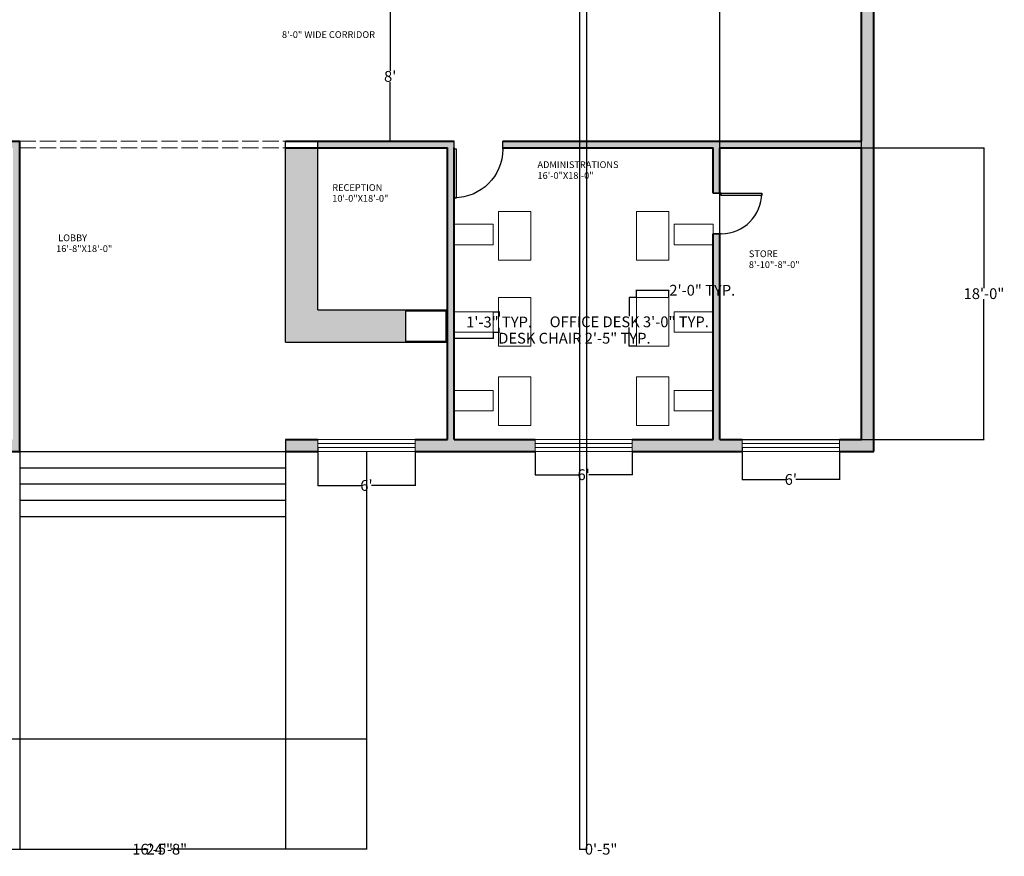
# Model space of a CAD drawing. Units: inches. Extents: x -405 to 940, y 226 to 2032.
# Tile 2 of 10: x 183 to 913, y 226 to 846. Entities that reach past the tile are written whole.
import ezdxf

# ---------------------------------------------------------------- set-up
doc = ezdxf.new("R2010")
doc.units = ezdxf.units.IN
doc.header["$MEASUREMENT"] = 0
doc.linetypes.add('ACAD_ISO02W100', pattern=[15, 12, -3])
for name, color, linetype, lineweight in [('A-ANNO-DIMS', 120, 'Continuous', 18), ('A-AREA-IDEN', 32, 'Continuous', 18), ('A-DOOR-OVHD', 6, 'ACAD_ISO02W100', 18), ('A-FLOR-CASE', 3, 'Continuous', 30), ('A-FLOR-EDGE', 3, 'Continuous', 25), ('A-FURN-SEAT', 5, 'Continuous', 18), ('A-GLAZ-HIDN', 1, 'ACAD_ISO02W100', 18), ('A-WALL-PATT', 8, 'Continuous', 13), ('door', 6, 'Continuous', 25), ('stair', 38, 'Continuous', 25), ('tables', 2, 'Continuous', 18), ('wall', 3, 'Continuous', 40), ('window', 1, 'Continuous', 18)]:
    doc.layers.add(name, color=color, linetype=linetype, lineweight=lineweight)
doc.styles.get("Standard").update_dxf_attribs({"font": 'arial.ttf'})
doc.dimstyles.get("Standard").update_dxf_attribs({"dimtxt": 8, "dimasz": 0.18, "dimexe": 0.18, "dimexo": 0.0625, "dimgap": 0.09, "dimtad": 0, "dimtih": 1, "dimtoh": 1, "dimdec": 0, "dimzin": 0, "dimdsep": 46, "dimlunit": 3, "dimtxsty": 'Standard', "dimblk": 'OBLIQUE', "dimcen": 0.09, "dimadec": 0, "dimazin": 0, "dimtfac": 1, "dimtdec": 0, "dimtofl": 0, "dimtmove": 0, "dimatfit": 3, "dimfxl": 1, "dimtolj": 1, "dimtzin": 0, "dimarcsym": 0})

# ---------------------------------------------------------------- blocks, each defined once
blk = doc.blocks.new('*U3')
for p, q in [((0, 0), (0, -6)), ((30, 0), (30, -6))]:
    blk.add_line(p, q)
blk.add_lwpolyline([(0, 0), (0, 30), (1.75, 30), (1.75, 0)], close=True)
blk.add_arc((0, 0), 30, 0, 90)
blk = doc.blocks.new('*U4')
for p, q in [((0, 0), (0, -6)), ((36, 0), (36, -6))]:
    blk.add_line(p, q)
blk.add_lwpolyline([(0, 0), (0, 36), (1.75, 36), (1.75, 0)], close=True)
blk.add_arc((0, 0), 36, 0, 90)
blk = doc.blocks.new('_Oblique')
at = {"color": 0, "linetype": 'ByBlock', "lineweight": -2}
blk.add_line((-0.5, -0.5), (0.5, 0.5), dxfattribs=at)
blk = doc.blocks.new('*D39')
at = {"layer": 'A-ANNO-DIMS', "color": 0, "lineweight": -2, "transparency": 16777216}
for p, q in [((460.94, 851.81), (457.18, 851.81)), ((457.36, 851.81), (457.36, 807.98)), ((457.36, 755.81), (457.36, 799.64)), ((460.94, 755.81), (457.18, 755.81))]:
    blk.add_line(p, q, dxfattribs=at)
at = {"layer": 'Defpoints', "color": 0, "transparency": 16777216}
for p in [(457.36, 851.81), (461, 851.81), (461, 755.81)]:
    blk.add_point(p, dxfattribs=at)
at = {"layer": 'A-ANNO-DIMS', "color": 0, "lineweight": -2, "transparency": 16777216, "xscale": 0.18, "yscale": 0.18, "zscale": 0.18}
for p, rotation in [((457.36, 851.81), 90), ((457.36, 755.81), 270)]:
    blk.add_blockref('_Oblique', p, dxfattribs=dict(at, rotation=rotation))
at = {"layer": 'A-ANNO-DIMS', "color": 0, "transparency": 16777216, "insert": (457.36, 803.81), "char_height": 8, "attachment_point": 5}
blk.add_mtext("\\A1;8'", dxfattribs=at)
blk = doc.blocks.new('*D72')
at = {"layer": 'A-ANNO-DIMS', "color": 0, "lineweight": -2, "transparency": 16777216}
for p, q in [((718.27, 528.75), (718.27, 504.97)), ((790.27, 525.75), (790.27, 504.97)), ((718.27, 505.15), (750.48, 505.15)), ((790.27, 505.15), (758.06, 505.15))]:
    blk.add_line(p, q, dxfattribs=at)
at = {"layer": 'Defpoints', "color": 0, "transparency": 16777216}
for p in [(718.27, 528.81), (790.27, 525.81), (718.27, 505.15)]:
    blk.add_point(p, dxfattribs=at)
at = {"layer": 'A-ANNO-DIMS', "color": 0, "lineweight": -2, "transparency": 16777216, "xscale": 0.18, "yscale": 0.18, "zscale": 0.18, "rotation": 180}
blk.add_blockref('_Oblique', (718.27, 505.15), dxfattribs=at)
at = {"layer": 'A-ANNO-DIMS', "color": 0, "lineweight": -2, "transparency": 16777216, "xscale": 0.18, "yscale": 0.18, "zscale": 0.18}
blk.add_blockref('_Oblique', (790.27, 505.15), dxfattribs=at)
at = {"layer": 'A-ANNO-DIMS', "color": 0, "transparency": 16777216, "insert": (754.27, 505.15), "char_height": 8, "attachment_point": 5}
blk.add_mtext("\\A1;6'", dxfattribs=at)
blk = doc.blocks.new('*D73')
at = {"layer": 'A-ANNO-DIMS', "color": 0, "lineweight": -2, "transparency": 16777216}
for p, q in [((564.77, 525.75), (564.77, 508.48)), ((636.77, 525.75), (636.77, 508.48)), ((564.77, 508.66), (596.98, 508.66)), ((636.77, 508.66), (604.56, 508.66))]:
    blk.add_line(p, q, dxfattribs=at)
at = {"layer": 'Defpoints', "color": 0, "transparency": 16777216}
for p in [(564.77, 525.81), (636.77, 525.81), (636.77, 508.66)]:
    blk.add_point(p, dxfattribs=at)
at = {"layer": 'A-ANNO-DIMS', "color": 0, "lineweight": -2, "transparency": 16777216, "xscale": 0.18, "yscale": 0.18, "zscale": 0.18, "rotation": 180}
blk.add_blockref('_Oblique', (564.77, 508.66), dxfattribs=at)
at = {"layer": 'A-ANNO-DIMS', "color": 0, "lineweight": -2, "transparency": 16777216, "xscale": 0.18, "yscale": 0.18, "zscale": 0.18}
blk.add_blockref('_Oblique', (636.77, 508.66), dxfattribs=at)
at = {"layer": 'A-ANNO-DIMS', "color": 0, "transparency": 16777216, "insert": (600.77, 508.66), "char_height": 8, "attachment_point": 5}
blk.add_mtext("\\A1;6'", dxfattribs=at)
blk = doc.blocks.new('*D74')
at = {"layer": 'A-ANNO-DIMS', "color": 0, "lineweight": -2, "transparency": 16777216}
for p, q in [((403.77, 528.75), (403.77, 500.53)), ((475.77, 525.75), (475.77, 500.53)), ((403.77, 500.71), (435.98, 500.71)), ((475.77, 500.71), (443.56, 500.71))]:
    blk.add_line(p, q, dxfattribs=at)
at = {"layer": 'Defpoints', "color": 0, "transparency": 16777216}
for p in [(403.77, 528.81), (475.77, 525.81), (475.77, 500.71)]:
    blk.add_point(p, dxfattribs=at)
at = {"layer": 'A-ANNO-DIMS', "color": 0, "lineweight": -2, "transparency": 16777216, "xscale": 0.18, "yscale": 0.18, "zscale": 0.18, "rotation": 180}
blk.add_blockref('_Oblique', (403.77, 500.71), dxfattribs=at)
at = {"layer": 'A-ANNO-DIMS', "color": 0, "lineweight": -2, "transparency": 16777216, "xscale": 0.18, "yscale": 0.18, "zscale": 0.18}
blk.add_blockref('_Oblique', (475.77, 500.71), dxfattribs=at)
at = {"layer": 'A-ANNO-DIMS', "color": 0, "transparency": 16777216, "insert": (439.77, 500.71), "char_height": 8, "attachment_point": 5}
blk.add_mtext("\\A1;6'", dxfattribs=at)
blk = doc.blocks.new('DESK-24X36IN')
for p, q in [((0, 36), (24, 36)), ((0, 0), (0, 36)), ((24, 36), (24, 0)), ((24, 0), (0, 0))]:
    blk.add_line(p, q)
blk = doc.blocks.new('CHAIR-DESK')
blk.add_lwpolyline([(0, 15.21), (28.97, 15.21), (28.97, 0), (0, 0)], close=True)
blk = doc.blocks.new('WIN-PANE-72IN')
for p, q in [((0, 3), (72, 3)), ((0, 0), (72, 0))]:
    blk.add_line(p, q)
blk = doc.blocks.new('*D87')
at = {"layer": 'A-ANNO-DIMS', "color": 0, "lineweight": -2, "transparency": 16777216}
for p, q in [((504.77, 614.1), (504.77, 609.63)), ((533.73, 614.1), (533.73, 609.63)), ((504.77, 609.81), (533.73, 609.81)), ((533.73, 609.81), (533.91, 609.81))]:
    blk.add_line(p, q, dxfattribs=at)
at = {"layer": 'Defpoints', "color": 0, "transparency": 16777216}
for p in [(504.77, 614.16), (533.73, 614.16), (533.73, 609.81)]:
    blk.add_point(p, dxfattribs=at)
at = {"layer": 'A-ANNO-DIMS', "color": 0, "lineweight": -2, "transparency": 16777216, "xscale": 0.18, "yscale": 0.18, "zscale": 0.18, "rotation": 180}
blk.add_blockref('_Oblique', (504.77, 609.81), dxfattribs=at)
at = {"layer": 'A-ANNO-DIMS', "color": 0, "lineweight": -2, "transparency": 16777216, "xscale": 0.18, "yscale": 0.18, "zscale": 0.18}
blk.add_blockref('_Oblique', (533.73, 609.81), dxfattribs=at)
at = {"layer": 'A-ANNO-DIMS', "color": 0, "transparency": 16777216, "insert": (593.9, 609.81), "char_height": 8, "attachment_point": 5}
blk.add_mtext('\\A1;DESK CHAIR 2\'-5" TYP.', dxfattribs=at)
blk = doc.blocks.new('*D88')
at = {"layer": 'A-ANNO-DIMS', "color": 0, "lineweight": -2, "transparency": 16777216}
for p, q in [((533.8, 629.37), (538.26, 629.37)), ((538.08, 629.37), (538.08, 625.94)), ((533.8, 614.16), (538.26, 614.16)), ((538.08, 614.16), (538.08, 617.59))]:
    blk.add_line(p, q, dxfattribs=at)
at = {"layer": 'Defpoints', "color": 0, "transparency": 16777216}
for p in [(533.73, 629.37), (538.08, 629.37), (533.73, 614.16)]:
    blk.add_point(p, dxfattribs=at)
at = {"layer": 'A-ANNO-DIMS', "color": 0, "lineweight": -2, "transparency": 16777216, "xscale": 0.18, "yscale": 0.18, "zscale": 0.18}
for p, rotation in [((538.08, 629.37), 90), ((538.08, 614.16), 270)]:
    blk.add_blockref('_Oblique', p, dxfattribs=dict(at, rotation=rotation))
at = {"layer": 'A-ANNO-DIMS', "color": 0, "transparency": 16777216, "insert": (538.08, 621.77), "char_height": 8, "attachment_point": 5}
blk.add_mtext('\\A1;1\'-3" TYP.', dxfattribs=at)
blk = doc.blocks.new('*D89')
at = {"layer": 'A-ANNO-DIMS', "color": 0, "lineweight": -2, "transparency": 16777216}
for p, q in [((639.86, 639.95), (634.35, 639.95)), ((634.53, 639.95), (634.53, 626.19)), ((634.53, 603.95), (634.53, 617.72)), ((639.86, 603.95), (634.35, 603.95))]:
    blk.add_line(p, q, dxfattribs=at)
at = {"layer": 'Defpoints', "color": 0, "transparency": 16777216}
for p in [(634.53, 639.95), (639.93, 639.95), (639.93, 603.95)]:
    blk.add_point(p, dxfattribs=at)
at = {"layer": 'A-ANNO-DIMS', "color": 0, "lineweight": -2, "transparency": 16777216, "xscale": 0.18, "yscale": 0.18, "zscale": 0.18}
for p, rotation in [((634.53, 639.95), 90), ((634.53, 603.95), 270)]:
    blk.add_blockref('_Oblique', p, dxfattribs=dict(at, rotation=rotation))
at = {"layer": 'A-ANNO-DIMS', "color": 0, "transparency": 16777216, "insert": (634.53, 621.95), "char_height": 8, "attachment_point": 5}
blk.add_mtext('\\A1;OFFICE DESK 3\'-0" TYP.', dxfattribs=at)
blk = doc.blocks.new('*D90')
at = {"layer": 'A-ANNO-DIMS', "color": 0, "lineweight": -2, "transparency": 16777216}
for p, q in [((639.93, 640.02), (639.93, 645.53)), ((639.93, 645.35), (663.93, 645.35)), ((663.93, 640.02), (663.93, 645.53)), ((663.93, 645.35), (664.11, 645.35))]:
    blk.add_line(p, q, dxfattribs=at)
at = {"layer": 'Defpoints', "color": 0, "transparency": 16777216}
for p in [(663.93, 645.35), (639.93, 639.95), (663.93, 639.95)]:
    blk.add_point(p, dxfattribs=at)
at = {"layer": 'A-ANNO-DIMS', "color": 0, "lineweight": -2, "transparency": 16777216, "xscale": 0.18, "yscale": 0.18, "zscale": 0.18, "rotation": 180}
blk.add_blockref('_Oblique', (639.93, 645.35), dxfattribs=at)
at = {"layer": 'A-ANNO-DIMS', "color": 0, "lineweight": -2, "transparency": 16777216, "xscale": 0.18, "yscale": 0.18, "zscale": 0.18}
blk.add_blockref('_Oblique', (663.93, 645.35), dxfattribs=at)
at = {"layer": 'A-ANNO-DIMS', "color": 0, "transparency": 16777216, "insert": (688.65, 645.35), "char_height": 8, "attachment_point": 5}
blk.add_mtext('\\A1;2\'-0" TYP.', dxfattribs=at)
blk = doc.blocks.new('*D97')
at = {"layer": 'A-ANNO-DIMS', "color": 0, "lineweight": -2, "transparency": 16777216}
for p, q in [((143.77, 312.75), (143.77, 230.98)), ((439.77, 312.75), (439.77, 230.98)), ((143.77, 231.16), (277.87, 231.16)), ((439.77, 231.16), (305.67, 231.16))]:
    blk.add_line(p, q, dxfattribs=at)
at = {"layer": 'Defpoints', "color": 0, "transparency": 16777216}
for p in [(143.77, 312.81), (439.77, 312.81), (439.77, 231.16)]:
    blk.add_point(p, dxfattribs=at)
at = {"layer": 'A-ANNO-DIMS', "color": 0, "lineweight": -2, "transparency": 16777216, "xscale": 0.18, "yscale": 0.18, "zscale": 0.18, "rotation": 180}
blk.add_blockref('_Oblique', (143.77, 231.16), dxfattribs=at)
at = {"layer": 'A-ANNO-DIMS', "color": 0, "lineweight": -2, "transparency": 16777216, "xscale": 0.18, "yscale": 0.18, "zscale": 0.18}
blk.add_blockref('_Oblique', (439.77, 231.16), dxfattribs=at)
at = {"layer": 'A-ANNO-DIMS', "color": 0, "transparency": 16777216, "insert": (291.77, 231.16), "char_height": 8, "attachment_point": 5}
blk.add_mtext('\\A1;24\'-8"', dxfattribs=at)
blk = doc.blocks.new('*D110')
at = {"layer": 'A-ANNO-DIMS', "color": 0, "lineweight": -2, "transparency": 16777216}
for p, q in [((182.77, 477.75), (182.77, 230.98)), ((379.77, 477.75), (379.77, 230.98)), ((182.77, 231.16), (267.81, 231.16)), ((379.77, 231.16), (294.72, 231.16))]:
    blk.add_line(p, q, dxfattribs=at)
at = {"layer": 'Defpoints', "color": 0, "transparency": 16777216}
for p in [(182.77, 477.81), (379.77, 477.81), (379.77, 231.16)]:
    blk.add_point(p, dxfattribs=at)
at = {"layer": 'A-ANNO-DIMS', "color": 0, "lineweight": -2, "transparency": 16777216, "xscale": 0.18, "yscale": 0.18, "zscale": 0.18, "rotation": 180}
blk.add_blockref('_Oblique', (182.77, 231.16), dxfattribs=at)
at = {"layer": 'A-ANNO-DIMS', "color": 0, "lineweight": -2, "transparency": 16777216, "xscale": 0.18, "yscale": 0.18, "zscale": 0.18}
blk.add_blockref('_Oblique', (379.77, 231.16), dxfattribs=at)
at = {"layer": 'A-ANNO-DIMS', "color": 0, "transparency": 16777216, "insert": (281.27, 231.16), "char_height": 8, "attachment_point": 5}
blk.add_mtext('\\A1;16\'-5"', dxfattribs=at)
blk = doc.blocks.new('*D112')
at = {"layer": 'A-ANNO-DIMS', "color": 0, "lineweight": -2, "transparency": 16777216}
for p, q in [((701.77, 534.87), (701.77, 2020.64)), ((701.77, 2020.46), (743.54, 2020.46)), ((806.77, 2020.46), (765, 2020.46)), ((806.77, 534.87), (806.77, 2020.64))]:
    blk.add_line(p, q, dxfattribs=at)
at = {"layer": 'Defpoints', "color": 0, "transparency": 16777216}
for p in [(701.77, 2020.46), (701.77, 534.81), (806.77, 534.81)]:
    blk.add_point(p, dxfattribs=at)
at = {"layer": 'A-ANNO-DIMS', "color": 0, "lineweight": -2, "transparency": 16777216, "xscale": 0.18, "yscale": 0.18, "zscale": 0.18, "rotation": 180}
blk.add_blockref('_Oblique', (701.77, 2020.46), dxfattribs=at)
at = {"layer": 'A-ANNO-DIMS', "color": 0, "lineweight": -2, "transparency": 16777216, "xscale": 0.18, "yscale": 0.18, "zscale": 0.18}
blk.add_blockref('_Oblique', (806.77, 2020.46), dxfattribs=at)
at = {"layer": 'A-ANNO-DIMS', "color": 0, "transparency": 16777216, "insert": (754.27, 2020.46), "char_height": 8, "attachment_point": 5}
blk.add_mtext('\\A1;8\'-9"', dxfattribs=at)
blk = doc.blocks.new('*D113')
at = {"layer": 'A-ANNO-DIMS', "color": 0, "lineweight": -2, "transparency": 16777216}
for p, q in [((701.83, 750.81), (897.6, 750.81)), ((897.42, 750.81), (897.42, 646.98)), ((897.42, 534.81), (897.42, 638.64)), ((701.83, 534.81), (897.6, 534.81))]:
    blk.add_line(p, q, dxfattribs=at)
at = {"layer": 'Defpoints', "color": 0, "transparency": 16777216}
for p in [(701.77, 750.81), (897.42, 750.81), (701.77, 534.81)]:
    blk.add_point(p, dxfattribs=at)
at = {"layer": 'A-ANNO-DIMS', "color": 0, "lineweight": -2, "transparency": 16777216, "xscale": 0.18, "yscale": 0.18, "zscale": 0.18}
for p, rotation in [((897.42, 750.81), 90), ((897.42, 534.81), 270)]:
    blk.add_blockref('_Oblique', p, dxfattribs=dict(at, rotation=rotation))
at = {"layer": 'A-ANNO-DIMS', "color": 0, "transparency": 16777216, "insert": (897.42, 642.81), "char_height": 8, "attachment_point": 5}
blk.add_mtext('\\A1;18\'-0"', dxfattribs=at)
blk = doc.blocks.new('*D116')
at = {"layer": 'A-ANNO-DIMS', "color": 0, "lineweight": -2, "transparency": 16777216}
for p, q in [((597.77, 1339.75), (597.77, 230.98)), ((602.77, 1339.75), (602.77, 230.98)), ((597.77, 231.16), (602.77, 231.16)), ((602.77, 231.16), (602.95, 231.16))]:
    blk.add_line(p, q, dxfattribs=at)
at = {"layer": 'Defpoints', "color": 0, "transparency": 16777216}
for p in [(597.77, 1339.81), (602.77, 1339.81), (602.77, 231.16)]:
    blk.add_point(p, dxfattribs=at)
at = {"layer": 'A-ANNO-DIMS', "color": 0, "lineweight": -2, "transparency": 16777216, "xscale": 0.18, "yscale": 0.18, "zscale": 0.18, "rotation": 180}
blk.add_blockref('_Oblique', (597.77, 231.16), dxfattribs=at)
at = {"layer": 'A-ANNO-DIMS', "color": 0, "lineweight": -2, "transparency": 16777216, "xscale": 0.18, "yscale": 0.18, "zscale": 0.18}
blk.add_blockref('_Oblique', (602.77, 231.16), dxfattribs=at)
at = {"layer": 'A-ANNO-DIMS', "color": 0, "transparency": 16777216, "insert": (613.67, 231.16), "char_height": 8, "attachment_point": 5}
blk.add_mtext('\\A1;0\'-5"', dxfattribs=at)

msp = doc.modelspace()

# ---------------------------------------------------------------- hatches: boundary and pattern name
at = {"layer": 'A-WALL-PATT'}
h = msp.add_hatch(dxfattribs=at)
h.set_pattern_fill('AR-HBONE', color=256)
h.set_pattern_definition([(45, (599.8442, 904.9158), (0, 5.656854), [12, -4]), (135, (602.6726, 907.744), (4e-16, 5.656854), [12, -4])])
h.paths.add_polyline_path([(-248.23, 1045.81), (-257.23, 1045.81), (-257.23, 964.81), (-248.23, 964.81)], flags=17)
h.paths.add_polyline_path([(-248.23, 851.81), (-39.23, 851.81), (-39.23, 856.81), (-44.23, 856.81), (-248.23, 856.81), (-248.23, 892.81), (-257.23, 892.81), (-257.23, 839.81), (-248.23, 839.81)])
h.paths.add_polyline_path([(-248.23, 750.81), (124.74, 750.81), (124.74, 751.73), (124.74, 755.81), (-248.23, 755.81), (-248.23, 767.81), (-257.23, 767.81), (-257.23, 726.81), (-248.23, 726.81)])
h.paths.add_polyline_path([(-248.23, 654.81), (-257.23, 654.81), (-257.23, 630.81), (-248.23, 630.81)])
h.paths.add_polyline_path([(-180.23, 534.81), (-248.23, 534.81), (-248.23, 558.81), (-257.23, 558.81), (-257.23, 525.81), (-180.23, 525.81)])
h.paths.add_polyline_path([(-69.23, 534.81), (-108.23, 534.81), (-108.23, 525.81), (-69.23, 525.81)])
h.paths.add_polyline_path([(35.77, 534.81), (2.77, 534.81), (2.77, 525.81), (35.77, 525.81)])
h.paths.add_polyline_path([(182.77, 755.81), (160.74, 755.81), (160.74, 750.81), (177.77, 750.81), (177.77, 534.81), (107.77, 534.81), (107.77, 525.81), (182.77, 525.81)])
h.paths.add_polyline_path([(-39.23, 1609.81), (-44.23, 1609.81), (-44.23, 1604.81), (-44.23, 1460.81), (-135.23, 1460.81), (-135.23, 1465.73), (-140.23, 1465.73), (-140.23, 1460.81), (-248.23, 1460.81), (-248.23, 1471.31), (-257.23, 1471.31), (-257.23, 1419.81), (-248.23, 1419.81), (-248.23, 1455.81), (-44.23, 1455.81), (-44.23, 1194.81), (-39.23, 1194.81)])
h.paths.add_polyline_path([(-248.23, 1520.81), (-257.23, 1520.81), (-257.23, 1495.31), (-248.23, 1495.31), (-248.23, 1505.81), (-140.23, 1505.81), (-140.23, 1495.73), (-135.23, 1495.73), (-135.23, 1516.79), (-140.23, 1516.79), (-140.23, 1510.81), (-248.23, 1510.81)], flags=17)
h.paths.add_polyline_path([(-248.23, 1570.31), (-257.23, 1570.31), (-257.23, 1544.81), (-248.23, 1544.81), (-248.23, 1554.81), (-140.23, 1554.81), (-140.23, 1546.79), (-135.23, 1546.79), (-135.23, 1565.08), (-140.23, 1565.08), (-140.23, 1559.81), (-248.23, 1559.81)], flags=17)
h.paths.add_polyline_path([(-248.23, 1615.81), (-257.23, 1615.81), (-257.23, 1594.31), (-248.23, 1594.31), (-248.23, 1604.81), (-140.23, 1604.81), (-140.23, 1595.08), (-135.23, 1595.08), (-135.23, 1604.81), (-80.23, 1604.81), (-80.23, 1609.81), (-248.23, 1609.81)])
h.paths.add_polyline_path([(-248.23, 1783.81), (-235.46, 1783.81), (-235.46, 1788.81), (-248.23, 1788.81), (-248.23, 1878.81), (-237.73, 1878.81), (-237.73, 1887.81), (-257.23, 1887.81), (-257.23, 1687.81), (-248.23, 1687.81), (-248.23, 1693.81), (-136.23, 1693.81), (-136.23, 1698.81), (-248.23, 1698.81)])
h.paths.add_polyline_path([(-188.23, 1887.81), (-213.73, 1887.81), (-213.73, 1878.81), (-203.23, 1878.81), (-203.23, 1788.81), (-205.46, 1788.81), (-205.46, 1783.81), (-186.39, 1783.81), (-186.39, 1788.81), (-198.23, 1788.81), (-198.23, 1878.81), (-188.23, 1878.81)])
h.paths.add_polyline_path([(-139.23, 1887.81), (-164.23, 1887.81), (-164.23, 1878.81), (-154.23, 1878.81), (-154.23, 1788.81), (-156.39, 1788.81), (-156.39, 1783.81), (-138.25, 1783.81), (-138.25, 1788.81), (-149.23, 1788.81), (-149.23, 1878.81), (-139.23, 1878.81)])
h.paths.add_polyline_path([(-89.23, 1887.81), (-115.23, 1887.81), (-115.23, 1878.81), (-105.23, 1878.81), (-105.23, 1788.81), (-108.25, 1788.81), (-108.25, 1783.81), (-86.45, 1783.81), (-86.45, 1788.81), (-100.23, 1788.81), (-100.23, 1878.81), (-89.23, 1878.81)])
h.paths.add_polyline_path([(-36.23, 1887.81), (-65.23, 1887.81), (-65.23, 1878.81), (-54.23, 1878.81), (-54.23, 1788.81), (-56.45, 1788.81), (-56.45, 1783.81), (-54.23, 1783.81), (-54.23, 1698.81), (-100.23, 1698.81), (-100.23, 1693.81), (-49.23, 1693.81), (-49.23, 1698.81), (-49.23, 1878.81), (-36.23, 1878.81)])
h.paths.add_polyline_path([(89.77, 1887.81), (35.77, 1887.81), (35.77, 1878.81), (48.77, 1878.81), (48.77, 1698.81), (-13.23, 1698.81), (-13.23, 1693.81), (53.77, 1693.81), (53.77, 1698.81), (53.77, 1878.81), (89.77, 1878.81)])
h.paths.add_polyline_path([(255.27, 1887.81), (161.77, 1887.81), (161.77, 1878.81), (197.77, 1878.81), (197.77, 1698.81), (89.77, 1698.81), (89.77, 1693.81), (202.77, 1693.81), (202.77, 1698.81), (202.77, 1878.81), (255.27, 1878.81)])
h.paths.add_polyline_path([(375.27, 1887.81), (327.27, 1887.81), (327.27, 1878.81), (375.27, 1878.81)], flags=17)
h.paths.add_polyline_path([(815.77, 1887.81), (447.27, 1887.81), (447.27, 1878.81), (499.77, 1878.81), (499.77, 1698.81), (238.77, 1698.81), (238.77, 1693.81), (504.77, 1693.81), (504.77, 1878.81), (633.77, 1878.81), (633.77, 1646.81), (597.77, 1646.81), (597.77, 1641.81), (602.77, 1641.81), (638.77, 1641.81), (638.77, 1878.81), (806.77, 1878.81), (806.77, 1838.31), (815.77, 1838.31)])
h.paths.add_polyline_path([(815.77, 1766.31), (806.77, 1766.31), (806.77, 1718.31), (815.77, 1718.31)], flags=17)
h.paths.add_polyline_path([(815.77, 1356.31), (806.77, 1356.31), (806.77, 1303.81), (602.77, 1303.81), (597.77, 1303.81), (597.77, 1037.81), (602.77, 1037.81), (602.77, 1298.81), (806.77, 1298.81), (806.77, 1246.31), (815.77, 1246.31)])
h.paths.add_polyline_path([(815.77, 1174.31), (806.77, 1174.31), (806.77, 1126.31), (815.77, 1126.31)], flags=17)
h.paths.add_polyline_path([(815.77, 1054.31), (806.77, 1054.31), (806.77, 1001.81), (796.08, 1001.81), (796.08, 1001.75), (780.86, 1001.75), (602.77, 1001.81), (597.77, 1001.81), (597.77, 892.81), (602.77, 892.81), (602.77, 996.81), (806.77, 996.81), (806.77, 962.81), (815.77, 962.81)])
h.paths.add_polyline_path([(403.77, 534.81), (379.77, 534.81), (379.77, 525.81), (403.77, 525.81)])
h.paths.add_polyline_path([(-39.23, 1158.81), (-44.23, 1158.81), (-248.23, 1158.81), (-248.23, 1194.81), (-257.23, 1194.81), (-257.23, 1117.81), (-248.23, 1117.81), (-248.23, 1153.81), (-44.23, 1153.81), (-44.23, 892.81), (-39.23, 892.81)])
h.paths.add_polyline_path([(-248.23, 1347.81), (-257.23, 1347.81), (-257.23, 1275.81), (-248.23, 1275.81)], flags=17)
h.paths.add_polyline_path([(815.77, 1476.31), (806.77, 1476.31), (806.77, 1428.31), (815.77, 1428.31)], flags=17)
h.paths.add_polyline_path([(815.77, 1646.31), (806.77, 1646.31), (806.77, 1638.65), (806.77, 1605.81), (597.77, 1605.81), (597.77, 1339.81), (602.77, 1339.81), (602.77, 1600.81), (806.77, 1600.81), (806.77, 1548.31), (815.77, 1548.31)])
h = msp.add_hatch(dxfattribs=at)
h.set_pattern_fill('AR-HBONE', color=256, scale=1.25)
h.paths.add_polyline_path([(815.77, 890.81), (806.77, 890.81), (806.77, 856.81), (602.77, 856.81), (597.77, 856.81), (597.77, 851.81), (806.77, 851.81), (806.77, 755.81), (540.77, 755.81), (540.77, 750.81), (696.77, 750.81), (696.77, 717.23), (701.77, 717.23), (701.77, 750.81), (806.77, 750.81), (806.77, 534.81), (790.27, 534.81), (790.27, 525.81), (815.77, 525.81)])
h.paths.add_polyline_path([(718.27, 534.81), (701.77, 534.81), (701.77, 687.23), (696.77, 687.23), (696.77, 679), (696.77, 534.81), (636.77, 534.81), (636.77, 525.81), (718.27, 525.81)], flags=17)
h.paths.add_polyline_path([(564.77, 534.81), (504.77, 534.81), (504.77, 750.81), (504.77, 755.81), (403.77, 755.81), (403.77, 750.81), (499.77, 750.81), (499.77, 534.81), (475.77, 534.81), (475.77, 525.81), (564.77, 525.81)])
h.paths.add_polyline_path([(499.77, 630.81), (403.77, 630.81), (403.77, 750.81), (379.77, 750.81), (379.77, 606.81), (499.77, 606.81)])
h.paths.add_polyline_path([(468.77, 629.86), (498.88, 629.86), (498.88, 607.6), (468.77, 607.6)], flags=16)
h.paths.add_polyline_path([(208.5, 672.29), (251.3, 672.29), (251.3, 679.95), (208.5, 679.95)], flags=9)
h.paths.add_polyline_path([(208.49, 680.3), (238.25, 680.3), (238.25, 688.06), (208.49, 688.06)], flags=9)

# ---------------------------------------------------------------- linework, layer by layer
at = {"layer": 'A-DOOR-OVHD'}
for p, q in [((182.77, 755.81), (379.77, 755.81)), ((182.77, 750.81), (379.77, 750.81))]:
    msp.add_line(p, q, dxfattribs=at)
at = {"layer": 'A-FLOR-CASE'}
for p, q in [((379.77, 606.81), (379.77, 755.81)), ((403.77, 630.81), (403.77, 755.81)), ((403.77, 630.81), (499.77, 630.81)), ((379.77, 606.81), (499.77, 606.81))]:
    msp.add_line(p, q, dxfattribs=at)
msp.add_lwpolyline([(498.88, 629.86), (468.77, 629.86), (468.77, 607.6), (498.88, 607.6)], close=True, dxfattribs=at)
at = {"layer": 'A-FLOR-EDGE'}
for p, q in [((439.77, 525.81), (439.77, 312.81)), ((439.77, 312.81), (143.77, 312.81))]:
    msp.add_line(p, q, dxfattribs=at)
at = {"layer": 'A-FURN-SEAT'}
msp.add_lwpolyline([(696.77, 694.21), (667.8, 694.21), (667.8, 679), (696.77, 679)], close=True, dxfattribs=at)
at = {"layer": 'A-GLAZ-HIDN'}
for p, q in [((403.77, 534.81), (403.77, 525.81)), ((475.77, 534.81), (475.77, 525.81)), ((564.77, 534.81), (564.77, 525.81)), ((636.77, 534.81), (636.77, 525.81)), ((718.27, 534.81), (718.27, 525.81)), ((790.27, 534.81), (790.27, 525.81))]:
    msp.add_line(p, q, dxfattribs=at)
at = {"layer": 'door'}
for p, q in [((504.77, 750.81), (504.77, 755.81)), ((540.77, 750.81), (540.77, 755.81)), ((696.77, 717.23), (701.77, 717.23)), ((696.77, 687.23), (701.77, 687.23))]:
    msp.add_line(p, q, dxfattribs=at)
at = {"layer": 'stair'}
for p, q in [((379.77, 534.81), (379.77, 477.81)), ((182.77, 525.81), (182.77, 477.81)), ((182.77, 525.81), (379.77, 525.81)), ((182.77, 513.81), (379.77, 513.81)), ((182.77, 501.81), (379.77, 501.81)), ((182.77, 489.81), (379.77, 489.81)), ((182.77, 477.81), (379.77, 477.81))]:
    msp.add_line(p, q, dxfattribs=at)
at = {"layer": 'wall'}
for p, q in [((815.77, 525.81), (815.77, 890.81)), ((806.77, 755.81), (806.77, 851.81)), ((160.74, 755.81), (182.77, 755.81)), ((182.77, 525.81), (182.77, 755.81)), ((379.77, 755.81), (504.77, 755.81)), ((540.77, 755.81), (806.77, 755.81)), ((379.77, 750.81), (499.77, 750.81)), ((499.77, 534.81), (499.77, 750.81)), ((504.77, 534.81), (504.77, 750.81)), ((540.77, 750.81), (696.77, 750.81)), ((696.77, 717.23), (696.77, 750.81)), ((701.77, 750.81), (806.77, 750.81)), ((701.77, 717.23), (701.77, 750.81)), ((806.77, 534.81), (806.77, 750.81)), ((696.77, 534.81), (696.77, 687.23)), ((701.77, 534.81), (701.77, 687.23)), ((379.77, 534.81), (403.77, 534.81)), ((475.77, 534.81), (499.77, 534.81)), ((504.77, 534.81), (564.77, 534.81)), ((636.77, 534.81), (696.77, 534.81)), ((701.77, 534.81), (718.27, 534.81)), ((790.27, 534.81), (806.77, 534.81)), ((107.77, 525.81), (182.77, 525.81)), ((379.77, 525.81), (403.77, 525.81)), ((475.77, 525.81), (564.77, 525.81)), ((636.77, 525.81), (718.27, 525.81)), ((790.27, 525.81), (815.77, 525.81))]:
    msp.add_line(p, q, dxfattribs=at)
at = {"layer": 'window'}
for p, q in [((475.77, 534.81), (403.77, 534.81)), ((636.77, 534.81), (564.77, 534.81)), ((790.27, 534.81), (718.27, 534.81)), ((475.77, 531.81), (403.77, 531.81)), ((475.77, 528.81), (403.77, 528.81)), ((475.77, 525.81), (403.77, 525.81)), ((636.77, 525.81), (564.77, 525.81)), ((790.27, 531.81), (718.27, 531.81)), ((790.27, 528.81), (718.27, 528.81)), ((790.27, 525.81), (718.27, 525.81))]:
    msp.add_line(p, q, dxfattribs=at)

# ---------------------------------------------------------------- block references
at = {"layer": 'A-FURN-SEAT'}
for p in [(504.77, 679), (504.77, 614.16), (504.77, 555.88)]:
    msp.add_blockref('CHAIR-DESK', p, dxfattribs=at)
at = {"layer": 'A-FURN-SEAT', "extrusion": (0, 0, -1), "zscale": -1}
for p in [(-696.77, 614.16), (-696.77, 555.88)]:
    msp.add_blockref('CHAIR-DESK', p, dxfattribs=at)
at = {"layer": 'door', "xscale": -1, "rotation": 180}
msp.add_blockref('*U4', (504.77, 749.81), dxfattribs=at)
at = {"layer": 'door', "rotation": 270}
msp.add_blockref('*U3', (702.77, 717.23), dxfattribs=at)
at = {"layer": 'tables'}
for p in [(537.61, 667.57), (639.93, 667.57), (537.61, 603.95), (639.93, 603.95), (537.61, 545.19), (639.93, 545.19)]:
    msp.add_blockref('DESK-24X36IN', p, dxfattribs=at)
at = {"layer": 'window'}
msp.add_blockref('WIN-PANE-72IN', (564.77, 528.81), dxfattribs=at)

# ---------------------------------------------------------------- texts
at = {"layer": 'A-AREA-IDEN'}
for s, p in [('8\'-0" WIDE CORRIDOR ', (377.13, 832.28)), ('ADMINISTRATIONS', (566.52, 735.89)), ('16\'-0"X18\'-0"', (566.52, 727.85)), ('RECEPTION ', (414.41, 718.94)), ('10\'-0"X18\'-0"', (414.41, 710.91)), (' LOBBY ', (209.78, 681.68)), ('16\'-8"X18\'-0"', (209.78, 673.65)), ('STORE ', (723.19, 669.86)), ('8\'-10"-8"-0"', (723.19, 661.83))]:
    msp.add_text(s, height=5, dxfattribs=at).set_placement(p)

# ---------------------------------------------------------------- dimensions: what is measured, and where the dimension line sits
at = {"layer": 'A-ANNO-DIMS'}
for base, p1, p2, override, picture, middle in [((701.77, 2020.46), (806.77, 534.81), (701.77, 534.81), {"dimdec": 1, "dimlfac": 1, "dimrnd": 0, "dimzin": 1, "dimdsep": 46, "dimlunit": 4, "dimfrac": 2}, '*D112', (754.27, 2020.46)), ((602.77, 231.16), (597.77, 1339.81), (602.77, 1339.81), {"dimdec": 1, "dimlfac": 1, "dimrnd": 0, "dimzin": 1, "dimdsep": 46, "dimlunit": 4, "dimfrac": 2}, '*D116', (613.67, 231.16)), ((475.77, 500.71), (403.77, 528.81), (475.77, 525.81), {"dimclrd": 0, "dimclre": 0, "dimclrt": 0}, '*D74', (439.77, 500.71)), ((636.77, 508.66), (564.77, 525.81), (636.77, 525.81), {"dimclrd": 0, "dimclre": 0, "dimclrt": 0}, '*D73', (600.77, 508.66)), ((718.27, 505.15), (790.27, 525.81), (718.27, 528.81), {"dimclrd": 0, "dimclre": 0, "dimclrt": 0}, '*D72', (754.27, 505.15)), ((379.77, 231.16), (182.77, 477.81), (379.77, 477.81), {"dimdec": 1, "dimlfac": 1, "dimrnd": 0, "dimzin": 1, "dimdsep": 46, "dimlunit": 4, "dimfrac": 2}, '*D110', (281.27, 231.16)), ((439.77, 231.16), (143.77, 312.81), (439.77, 312.81), {"dimdec": 1, "dimlfac": 1, "dimrnd": 0, "dimzin": 1, "dimdsep": 46, "dimlunit": 4, "dimfrac": 2}, '*D97', (291.77, 231.16))]:
    dim = msp.add_linear_dim(base=base, p1=p1, p2=p2, dimstyle='Standard', override=override, dxfattribs=at)
    dim.commit()
    dim.dimension.update_dxf_attribs({"geometry": picture, "text_midpoint": middle})
for base, p1, p2, override, picture, middle in [((457.36, 851.81), (461, 755.81), (461, 851.81), {"dimclrd": 0, "dimclre": 0, "dimclrt": 0}, '*D39', (457.36, 803.81)), ((897.42, 750.81), (701.77, 534.81), (701.77, 750.81), {"dimdec": 1, "dimlfac": 1, "dimrnd": 0, "dimzin": 1, "dimdsep": 46, "dimlunit": 4, "dimfrac": 2}, '*D113', (897.42, 642.81))]:
    dim = msp.add_linear_dim(base=base, p1=p1, p2=p2, angle=90, dimstyle='Standard', override=override, dxfattribs=at)
    dim.commit()
    dim.dimension.update_dxf_attribs({"geometry": picture, "text_midpoint": middle})
for base, p1, p2, text, picture, middle in [((663.93, 645.35), (639.93, 639.95), (663.93, 639.95), '<> TYP.', '*D90', (688.65, 645.35)), ((533.73, 609.81), (504.77, 614.16), (533.73, 614.16), 'DESK CHAIR <> TYP.', '*D87', (593.9, 609.81))]:
    dim = msp.add_linear_dim(base=base, p1=p1, p2=p2, text=text, dimstyle='Standard', override={"dimdec": 1, "dimlfac": 1, "dimrnd": 0, "dimzin": 1, "dimdsep": 46, "dimlunit": 4, "dimfrac": 2}, dxfattribs=at)
    dim.commit()
    dim.dimension.update_dxf_attribs({"geometry": picture, "text_midpoint": middle})
for base, p1, p2, text, picture, middle in [((634.53, 639.95), (639.93, 603.95), (639.93, 639.95), 'OFFICE DESK <> TYP.', '*D89', (634.53, 621.95)), ((538.08, 629.37), (533.73, 614.16), (533.73, 629.37), '<> TYP.', '*D88', (538.08, 621.77))]:
    dim = msp.add_linear_dim(base=base, p1=p1, p2=p2, angle=90, text=text, dimstyle='Standard', override={"dimdec": 1, "dimlfac": 1, "dimrnd": 0, "dimzin": 1, "dimdsep": 46, "dimlunit": 4, "dimfrac": 2}, dxfattribs=at)
    dim.commit()
    dim.dimension.update_dxf_attribs({"geometry": picture, "text_midpoint": middle})

doc.saveas('drawing.dxf')
